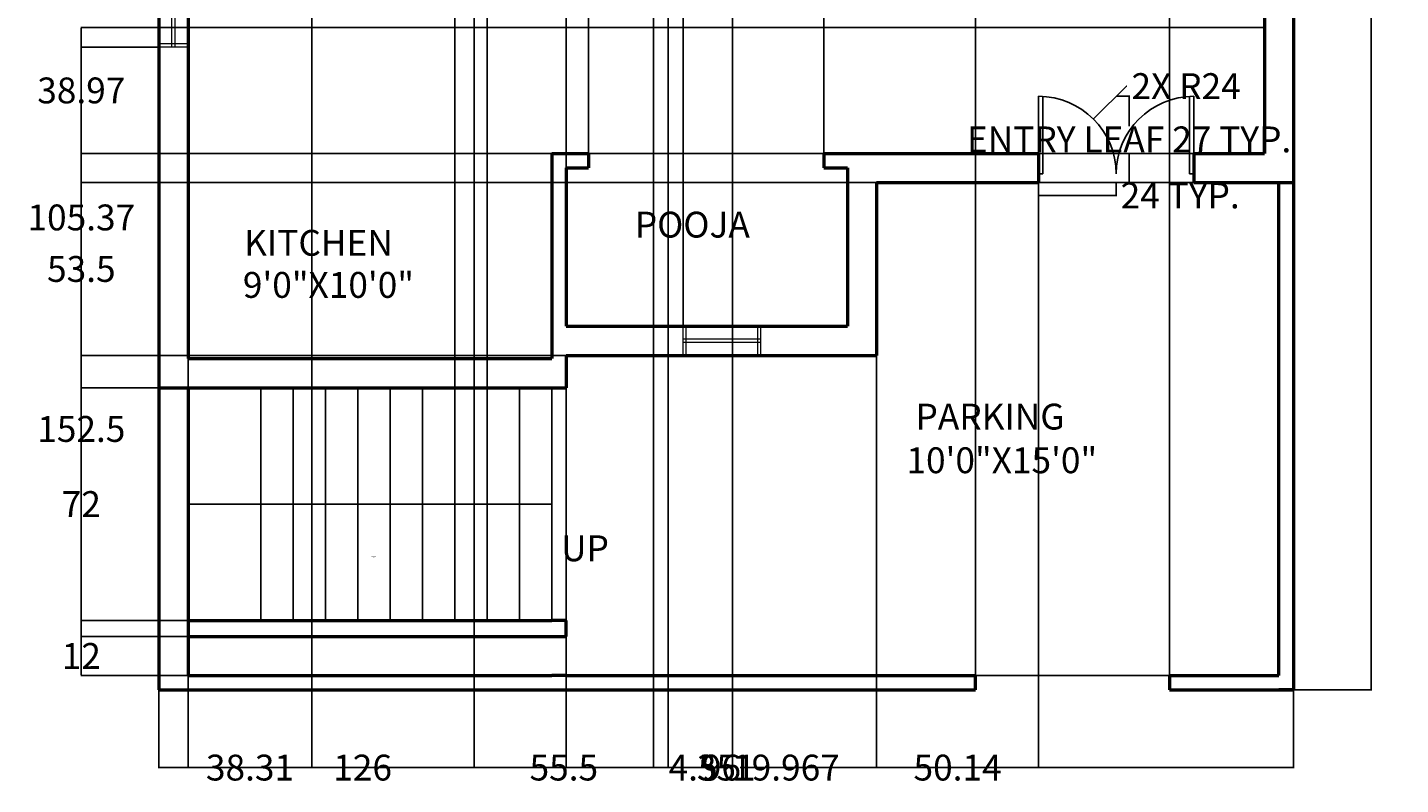
# Model space of a CAD drawing. Units: inches. Extents: x 16123781 to 16124206, y 158262361 to 158262900.
# Tile 1 of 2: x 16123781 to 16124206, y 158262361 to 158262596. Entities that reach past the tile are written whole.
import ezdxf

# ---------------------------------------------------------------- set-up
doc = ezdxf.new("R2010")
doc.units = ezdxf.units.IN
for name, color, linetype, lineweight in [('A-ANNO-DIMS', 2, 'Continuous', 18), ('A-ANNO-SYMB', 7, 'Continuous', 18), ('A-ANNO-TEXT', 7, 'Continuous', 25), ('A-AREA-IDEN', 7, 'Continuous', 25), ('A-Door', 150, 'Continuous', 25), ('stair', 10, 'Continuous', 25), ('wall', 130, 'Continuous', 50), ('window', 80, 'Continuous', 18)]:
    doc.layers.add(name, color=color, linetype=linetype, lineweight=lineweight)
doc.styles.get("Standard").update_dxf_attribs({"font": 'arial.ttf', "height": 8})
doc.dimstyles.get("Standard").update_dxf_attribs({"dimtxt": 0.18, "dimasz": 0.18, "dimexe": 0.18, "dimexo": 0.0625, "dimgap": 0.09, "dimtad": 0, "dimtih": 1, "dimtoh": 1, "dimdec": 4, "dimzin": 0, "dimdsep": 46, "dimtxsty": 'Standard', "dimcen": 0.09, "dimadec": 0, "dimazin": 0, "dimtfac": 1, "dimtdec": 4, "dimtofl": 0, "dimtmove": 0, "dimatfit": 3, "dimfxl": 1, "dimtolj": 1, "dimtzin": 0, "dimarcsym": 0})

# ---------------------------------------------------------------- blocks, each defined once
blk = doc.blocks.new('WIN-48IN')
for p, q in [((0, 0), (0, 48)), ((0, 48), (9, 48)), ((0, 47), (9, 47)), ((4, 0), (4, 48)), ((5, 0), (5, 48)), ((9, 48), (9, 0)), ((9, 1), (0, 1)), ((9, 0), (0, 0))]:
    blk.add_line(p, q)
blk = doc.blocks.new('WIN-24IN')
for p, q in [((0, 9), (24, 9)), ((0, 0), (0, 9)), ((1, 0), (1, 9)), ((23, 9), (23, 0)), ((24, 9), (24, 0)), ((24, 5), (0, 5)), ((24, 4), (0, 4)), ((24, 0), (0, 0))]:
    blk.add_line(p, q)
blk = doc.blocks.new('DOOR-LEAF-24IN')
for p, q in [((0, 0), (0, 26.67)), ((1.33, 2.67), (1.33, 26.63)), ((0, 2.67), (1.33, 2.67)), ((0, 0), (0, 1.6))]:
    blk.add_line(p, q)
blk.add_arc((0, 2.67), 24, 0, 90)
blk = doc.blocks.new('*D15')
at = {"layer": 'A-ANNO-DIMS', "color": 0, "lineweight": -2, "transparency": 16777216}
for p, q in [((16124117.96, 158262574.23), (16124122.08, 158262574.23)), ((16124121.9, 158262574.05), (16124121.9, 158262565.01)), ((16124121.9, 158262547.74), (16124121.9, 158262556.79)), ((16124117.96, 158262547.56), (16124122.08, 158262547.56))]:
    blk.add_line(p, q, dxfattribs=at)
at = {"layer": 'A-ANNO-DIMS', "color": 0, "transparency": 16777216}
for points in [[(16124121.87, 158262574.05), (16124121.93, 158262574.05), (16124121.9, 158262574.23)], [(16124121.87, 158262547.74), (16124121.93, 158262547.74), (16124121.9, 158262547.56)]]:
    blk.add_solid(points, dxfattribs=at)
at = {"layer": 'Defpoints', "color": 0, "transparency": 16777216}
for p in [(16124117.9, 158262574.23), (16124121.9, 158262574.23), (16124117.9, 158262547.56)]:
    blk.add_point(p, dxfattribs=at)
at = {"layer": 'A-ANNO-DIMS', "color": 0, "transparency": 16777216, "insert": (16124121.9, 158262560.9), "char_height": 8, "attachment_point": 5}
blk.add_mtext('\\A1;ENTRY LEAF 27 TYP.', dxfattribs=at)
blk = doc.blocks.new('*D16')
at = {"layer": 'A-ANNO-DIMS', "color": 0, "lineweight": -2, "transparency": 16777216}
for p, q in [((16124093.9, 158262547.5), (16124093.9, 158262543.38)), ((16124117.9, 158262547.5), (16124117.9, 158262543.38)), ((16124094.08, 158262543.56), (16124117.72, 158262543.56)), ((16124117.9, 158262543.56), (16124118.08, 158262543.56))]:
    blk.add_line(p, q, dxfattribs=at)
at = {"layer": 'A-ANNO-DIMS', "color": 0, "transparency": 16777216}
for points in [[(16124094.08, 158262543.59), (16124094.08, 158262543.53), (16124093.9, 158262543.56)], [(16124117.72, 158262543.59), (16124117.72, 158262543.53), (16124117.9, 158262543.56)]]:
    blk.add_solid(points, dxfattribs=at)
at = {"layer": 'Defpoints', "color": 0, "transparency": 16777216}
for p in [(16124093.9, 158262547.56), (16124117.9, 158262547.56), (16124117.9, 158262543.56)]:
    blk.add_point(p, dxfattribs=at)
at = {"layer": 'A-ANNO-DIMS', "color": 0, "transparency": 16777216, "insert": (16124137.71, 158262543.56), "char_height": 8, "attachment_point": 5}
blk.add_mtext('\\A1;24 TYP.', dxfattribs=at)
blk = doc.blocks.new('*D17')
at = {"layer": 'A-ANNO-DIMS', "color": 0, "lineweight": -2, "transparency": 16777216}
for p, q in [((16123821.76, 158262390.5), (16123821.76, 158262366.35)), ((16124172.76, 158262390.5), (16124172.76, 158262366.35)), ((16123821.94, 158262366.53), (16123989.11, 158262366.53)), ((16124172.58, 158262366.53), (16124005.41, 158262366.53))]:
    blk.add_line(p, q, dxfattribs=at)
at = {"layer": 'A-ANNO-DIMS', "color": 0, "transparency": 16777216}
for points in [[(16123821.94, 158262366.56), (16123821.94, 158262366.5), (16123821.76, 158262366.53)], [(16124172.58, 158262366.56), (16124172.58, 158262366.5), (16124172.76, 158262366.53)]]:
    blk.add_solid(points, dxfattribs=at)
at = {"layer": 'Defpoints', "color": 0, "transparency": 16777216}
for p in [(16123821.76, 158262390.56), (16124172.76, 158262390.56), (16124172.76, 158262366.53)]:
    blk.add_point(p, dxfattribs=at)
at = {"layer": 'A-ANNO-DIMS', "color": 0, "transparency": 16777216, "insert": (16123997.26, 158262366.53), "char_height": 8, "attachment_point": 5}
blk.add_mtext('\\A1;351', dxfattribs=at)
blk = doc.blocks.new('*D18')
at = {"layer": 'A-ANNO-DIMS', "color": 0, "lineweight": -2, "transparency": 16777216}
for p, q in [((16124172.82, 158262870.56), (16124196.97, 158262870.56)), ((16124196.79, 158262870.38), (16124196.79, 158262634.74)), ((16124196.79, 158262390.74), (16124196.79, 158262626.39)), ((16124172.82, 158262390.56), (16124196.97, 158262390.56))]:
    blk.add_line(p, q, dxfattribs=at)
at = {"layer": 'A-ANNO-DIMS', "color": 0, "transparency": 16777216}
for points in [[(16124196.76, 158262870.38), (16124196.82, 158262870.38), (16124196.79, 158262870.56)], [(16124196.76, 158262390.74), (16124196.82, 158262390.74), (16124196.79, 158262390.56)]]:
    blk.add_solid(points, dxfattribs=at)
at = {"layer": 'Defpoints', "color": 0, "transparency": 16777216}
for p in [(16124172.76, 158262870.56), (16124196.79, 158262870.56), (16124172.76, 158262390.56)]:
    blk.add_point(p, dxfattribs=at)
at = {"layer": 'A-ANNO-DIMS', "color": 0, "transparency": 16777216, "insert": (16124196.79, 158262630.56), "char_height": 8, "attachment_point": 5}
blk.add_mtext('\\A1;480', dxfattribs=at)
blk = doc.blocks.new('*D19')
at = {"layer": 'A-ANNO-DIMS', "color": 0, "lineweight": -2, "transparency": 16777216}
for p, q in [((16124074.35, 158262390.63), (16124074.35, 158262894.77)), ((16124074.53, 158262894.59), (16124098.52, 158262894.59)), ((16124134.17, 158262894.59), (16124110.18, 158262894.59)), ((16124134.35, 158262390.63), (16124134.35, 158262894.77))]:
    blk.add_line(p, q, dxfattribs=at)
at = {"layer": 'A-ANNO-DIMS', "color": 0, "transparency": 16777216}
for points in [[(16124074.53, 158262894.62), (16124074.53, 158262894.56), (16124074.35, 158262894.59)], [(16124134.17, 158262894.62), (16124134.17, 158262894.56), (16124134.35, 158262894.59)]]:
    blk.add_solid(points, dxfattribs=at)
at = {"layer": 'Defpoints', "color": 0, "transparency": 16777216}
for p in [(16124134.35, 158262894.59), (16124074.35, 158262390.56), (16124134.35, 158262390.56)]:
    blk.add_point(p, dxfattribs=at)
at = {"layer": 'A-ANNO-DIMS', "color": 0, "transparency": 16777216, "insert": (16124104.35, 158262894.59), "char_height": 8, "attachment_point": 5}
blk.add_mtext('\\A1;60', dxfattribs=at)
blk = doc.blocks.new('*D20')
at = {"layer": 'A-ANNO-DIMS', "color": 0, "lineweight": -2, "transparency": 16777216}
for p, q in [((16124134.35, 158262390.63), (16124134.35, 158262894.77)), ((16124134.53, 158262894.59), (16124140.74, 158262894.59)), ((16124172.58, 158262894.59), (16124166.37, 158262894.59)), ((16124172.76, 158262390.63), (16124172.76, 158262894.77))]:
    blk.add_line(p, q, dxfattribs=at)
at = {"layer": 'A-ANNO-DIMS', "color": 0, "transparency": 16777216}
for points in [[(16124134.53, 158262894.62), (16124134.53, 158262894.56), (16124134.35, 158262894.59)], [(16124172.58, 158262894.62), (16124172.58, 158262894.56), (16124172.76, 158262894.59)]]:
    blk.add_solid(points, dxfattribs=at)
at = {"layer": 'Defpoints', "color": 0, "transparency": 16777216}
for p in [(16124172.76, 158262894.59), (16124134.35, 158262390.56), (16124172.76, 158262390.56)]:
    blk.add_point(p, dxfattribs=at)
at = {"layer": 'A-ANNO-DIMS', "color": 0, "transparency": 16777216, "insert": (16124153.55, 158262894.59), "char_height": 8, "attachment_point": 5}
blk.add_mtext('\\A1;38.41', dxfattribs=at)
blk = doc.blocks.new('*D21')
at = {"layer": 'A-ANNO-DIMS', "color": 0, "lineweight": -2, "transparency": 16777216}
for p, q in [((16123821.76, 158262484), (16123821.76, 158262366.35)), ((16123947.76, 158262484), (16123947.76, 158262366.35)), ((16123821.94, 158262366.53), (16123876.21, 158262366.53)), ((16123947.58, 158262366.53), (16123893.31, 158262366.53))]:
    blk.add_line(p, q, dxfattribs=at)
at = {"layer": 'A-ANNO-DIMS', "color": 0, "transparency": 16777216}
for points in [[(16123821.94, 158262366.56), (16123821.94, 158262366.5), (16123821.76, 158262366.53)], [(16123947.58, 158262366.56), (16123947.58, 158262366.5), (16123947.76, 158262366.53)]]:
    blk.add_solid(points, dxfattribs=at)
at = {"layer": 'Defpoints', "color": 0, "transparency": 16777216}
for p in [(16123821.76, 158262484.06), (16123947.76, 158262484.06), (16123947.76, 158262366.53)]:
    blk.add_point(p, dxfattribs=at)
at = {"layer": 'A-ANNO-DIMS', "color": 0, "transparency": 16777216, "insert": (16123884.76, 158262366.53), "char_height": 8, "attachment_point": 5}
blk.add_mtext('\\A1;126', dxfattribs=at)
blk = doc.blocks.new('*D22')
at = {"layer": 'A-ANNO-DIMS', "color": 0, "lineweight": -2, "transparency": 16777216}
for p, q in [((16123947.76, 158262494), (16123947.76, 158262366.35)), ((16124043.76, 158262494), (16124043.76, 158262366.35)), ((16123947.94, 158262366.53), (16123989.94, 158262366.53)), ((16124043.58, 158262366.53), (16124001.58, 158262366.53))]:
    blk.add_line(p, q, dxfattribs=at)
at = {"layer": 'A-ANNO-DIMS', "color": 0, "transparency": 16777216}
for points in [[(16123947.94, 158262366.56), (16123947.94, 158262366.5), (16123947.76, 158262366.53)], [(16124043.58, 158262366.56), (16124043.58, 158262366.5), (16124043.76, 158262366.53)]]:
    blk.add_solid(points, dxfattribs=at)
at = {"layer": 'Defpoints', "color": 0, "transparency": 16777216}
for p in [(16123947.76, 158262494.06), (16124043.76, 158262494.06), (16124043.76, 158262366.53)]:
    blk.add_point(p, dxfattribs=at)
at = {"layer": 'A-ANNO-DIMS', "color": 0, "transparency": 16777216, "insert": (16123995.76, 158262366.53), "char_height": 8, "attachment_point": 5}
blk.add_mtext('\\A1;96', dxfattribs=at)
blk = doc.blocks.new('*D23')
at = {"layer": 'A-ANNO-DIMS', "color": 0, "lineweight": -2, "transparency": 16777216}
for p, q in [((16123947.76, 158262503.13), (16123947.76, 158262894.77)), ((16123947.94, 158262894.59), (16123952.22, 158262894.59)), ((16123983.73, 158262894.59), (16123979.45, 158262894.59)), ((16123983.91, 158262503.13), (16123983.91, 158262894.77))]:
    blk.add_line(p, q, dxfattribs=at)
at = {"layer": 'A-ANNO-DIMS', "color": 0, "transparency": 16777216}
for points in [[(16123947.94, 158262894.62), (16123947.94, 158262894.56), (16123947.76, 158262894.59)], [(16123983.73, 158262894.62), (16123983.73, 158262894.56), (16123983.91, 158262894.59)]]:
    blk.add_solid(points, dxfattribs=at)
at = {"layer": 'Defpoints', "color": 0, "transparency": 16777216}
for p in [(16123983.91, 158262894.59), (16123947.76, 158262503.06), (16123983.91, 158262503.06)]:
    blk.add_point(p, dxfattribs=at)
at = {"layer": 'A-ANNO-DIMS', "color": 0, "transparency": 16777216, "insert": (16123965.84, 158262894.59), "char_height": 8, "attachment_point": 5}
blk.add_mtext('\\A1;36.15', dxfattribs=at)
blk = doc.blocks.new('*D24')
at = {"layer": 'A-ANNO-DIMS', "color": 0, "lineweight": -2, "transparency": 16777216}
for p, q in [((16123830.7, 158262407.06), (16123797.55, 158262407.06)), ((16123797.73, 158262406.88), (16123797.73, 158262405.17)), ((16123797.73, 158262395.24), (16123797.73, 158262396.96)), ((16123830.7, 158262395.06), (16123797.55, 158262395.06))]:
    blk.add_line(p, q, dxfattribs=at)
at = {"layer": 'A-ANNO-DIMS', "color": 0, "transparency": 16777216}
for points in [[(16123797.7, 158262406.88), (16123797.76, 158262406.88), (16123797.73, 158262407.06)], [(16123797.7, 158262395.24), (16123797.76, 158262395.24), (16123797.73, 158262395.06)]]:
    blk.add_solid(points, dxfattribs=at)
at = {"layer": 'Defpoints', "color": 0, "transparency": 16777216}
for p in [(16123797.73, 158262407.06), (16123830.76, 158262407.06), (16123830.76, 158262395.06)]:
    blk.add_point(p, dxfattribs=at)
at = {"layer": 'A-ANNO-DIMS', "color": 0, "transparency": 16777216, "insert": (16123797.73, 158262401.06), "char_height": 8, "attachment_point": 5}
blk.add_mtext('\\A1;12', dxfattribs=at)
blk = doc.blocks.new('*D25')
at = {"layer": 'A-ANNO-DIMS', "color": 0, "lineweight": -2, "transparency": 16777216}
for p, q in [((16124043.7, 158262547.56), (16123797.55, 158262547.56)), ((16123797.73, 158262547.38), (16123797.73, 158262524.99)), ((16123797.73, 158262494.24), (16123797.73, 158262516.64)), ((16124043.7, 158262494.06), (16123797.55, 158262494.06))]:
    blk.add_line(p, q, dxfattribs=at)
at = {"layer": 'A-ANNO-DIMS', "color": 0, "transparency": 16777216}
for points in [[(16123797.7, 158262547.38), (16123797.76, 158262547.38), (16123797.73, 158262547.56)], [(16123797.7, 158262494.24), (16123797.76, 158262494.24), (16123797.73, 158262494.06)]]:
    blk.add_solid(points, dxfattribs=at)
at = {"layer": 'Defpoints', "color": 0, "transparency": 16777216}
for p in [(16123797.73, 158262547.56), (16124043.76, 158262547.56), (16124043.76, 158262494.06)]:
    blk.add_point(p, dxfattribs=at)
at = {"layer": 'A-ANNO-DIMS', "color": 0, "transparency": 16777216, "insert": (16123797.73, 158262520.81), "char_height": 8, "attachment_point": 5}
blk.add_mtext('\\A1;53.5', dxfattribs=at)
blk = doc.blocks.new('*D26')
at = {"layer": 'A-ANNO-DIMS', "color": 0, "lineweight": -2, "transparency": 16777216}
for p, q in [((16124168.2, 158262547.56), (16123797.55, 158262547.56)), ((16123797.73, 158262547.38), (16123797.73, 158262475.49)), ((16123797.73, 158262395.24), (16123797.73, 158262467.14)), ((16124168.2, 158262395.06), (16123797.55, 158262395.06))]:
    blk.add_line(p, q, dxfattribs=at)
at = {"layer": 'A-ANNO-DIMS', "color": 0, "transparency": 16777216}
for points in [[(16123797.7, 158262547.38), (16123797.76, 158262547.38), (16123797.73, 158262547.56)], [(16123797.7, 158262395.24), (16123797.76, 158262395.24), (16123797.73, 158262395.06)]]:
    blk.add_solid(points, dxfattribs=at)
at = {"layer": 'Defpoints', "color": 0, "transparency": 16777216}
for p in [(16123797.73, 158262547.56), (16124168.26, 158262547.56), (16124168.26, 158262395.06)]:
    blk.add_point(p, dxfattribs=at)
at = {"layer": 'A-ANNO-DIMS', "color": 0, "transparency": 16777216, "insert": (16123797.73, 158262471.31), "char_height": 8, "attachment_point": 5}
blk.add_mtext('\\A1;152.5', dxfattribs=at)
blk = doc.blocks.new('*D27')
at = {"layer": 'A-ANNO-DIMS', "color": 0, "lineweight": -2, "transparency": 16777216}
for p, q in [((16124043.76, 158262547.5), (16124043.76, 158262366.35)), ((16124093.9, 158262547.5), (16124093.9, 158262366.35)), ((16124043.94, 158262366.53), (16124055.26, 158262366.53)), ((16124093.72, 158262366.53), (16124082.4, 158262366.53))]:
    blk.add_line(p, q, dxfattribs=at)
at = {"layer": 'A-ANNO-DIMS', "color": 0, "transparency": 16777216}
for points in [[(16124043.94, 158262366.56), (16124043.94, 158262366.5), (16124043.76, 158262366.53)], [(16124093.72, 158262366.56), (16124093.72, 158262366.5), (16124093.9, 158262366.53)]]:
    blk.add_solid(points, dxfattribs=at)
at = {"layer": 'Defpoints', "color": 0, "transparency": 16777216}
for p in [(16124043.76, 158262547.56), (16124093.9, 158262547.56), (16124093.9, 158262366.53)]:
    blk.add_point(p, dxfattribs=at)
at = {"layer": 'A-ANNO-DIMS', "color": 0, "transparency": 16777216, "insert": (16124068.83, 158262366.53), "char_height": 8, "attachment_point": 5}
blk.add_mtext('\\A1;50.14', dxfattribs=at)
blk = doc.blocks.new('*D28')
at = {"layer": 'A-ANNO-DIMS', "color": 0, "lineweight": -2, "transparency": 16777216}
for p, q in [((16123821.7, 158262589.43), (16123797.55, 158262589.43)), ((16123797.73, 158262589.25), (16123797.73, 158262540.92)), ((16123797.73, 158262484.24), (16123797.73, 158262532.57)), ((16123821.7, 158262484.06), (16123797.55, 158262484.06))]:
    blk.add_line(p, q, dxfattribs=at)
at = {"layer": 'A-ANNO-DIMS', "color": 0, "transparency": 16777216}
for points in [[(16123797.7, 158262589.25), (16123797.76, 158262589.25), (16123797.73, 158262589.43)], [(16123797.7, 158262484.24), (16123797.76, 158262484.24), (16123797.73, 158262484.06)]]:
    blk.add_solid(points, dxfattribs=at)
at = {"layer": 'Defpoints', "color": 0, "transparency": 16777216}
for p in [(16123797.73, 158262589.43), (16123821.76, 158262589.43), (16123821.76, 158262484.06)]:
    blk.add_point(p, dxfattribs=at)
at = {"layer": 'A-ANNO-DIMS', "color": 0, "transparency": 16777216, "insert": (16123797.73, 158262536.75), "char_height": 8, "attachment_point": 5}
blk.add_mtext('\\A1;105.37', dxfattribs=at)
blk = doc.blocks.new('*D31')
at = {"layer": 'A-ANNO-DIMS', "color": 0, "lineweight": -2, "transparency": 16777216}
for p, q in [((16124163.7, 158262595.53), (16123797.55, 158262595.53)), ((16123797.73, 158262595.35), (16123797.73, 158262580.23)), ((16123797.73, 158262556.74), (16123797.73, 158262571.87)), ((16124163.7, 158262556.56), (16123797.55, 158262556.56))]:
    blk.add_line(p, q, dxfattribs=at)
at = {"layer": 'A-ANNO-DIMS', "color": 0, "transparency": 16777216}
for points in [[(16123797.7, 158262595.35), (16123797.76, 158262595.35), (16123797.73, 158262595.53)], [(16123797.7, 158262556.74), (16123797.76, 158262556.74), (16123797.73, 158262556.56)]]:
    blk.add_solid(points, dxfattribs=at)
at = {"layer": 'Defpoints', "color": 0, "transparency": 16777216}
for p in [(16123797.73, 158262595.53), (16124163.76, 158262595.53), (16124163.76, 158262556.56)]:
    blk.add_point(p, dxfattribs=at)
at = {"layer": 'A-ANNO-DIMS', "color": 0, "transparency": 16777216, "insert": (16123797.73, 158262576.05), "char_height": 8, "attachment_point": 5}
blk.add_mtext('\\A1;38.97', dxfattribs=at)
blk = doc.blocks.new('*D34')
at = {"layer": 'A-ANNO-DIMS', "color": 0, "lineweight": -2, "transparency": 16777216}
for p, q in [((16123830.7, 158262484.06), (16123797.55, 158262484.06)), ((16123797.73, 158262483.88), (16123797.73, 158262452.17)), ((16123797.73, 158262412.24), (16123797.73, 158262443.96)), ((16123830.7, 158262412.06), (16123797.55, 158262412.06))]:
    blk.add_line(p, q, dxfattribs=at)
at = {"layer": 'A-ANNO-DIMS', "color": 0, "transparency": 16777216}
for points in [[(16123797.7, 158262483.88), (16123797.76, 158262483.88), (16123797.73, 158262484.06)], [(16123797.7, 158262412.24), (16123797.76, 158262412.24), (16123797.73, 158262412.06)]]:
    blk.add_solid(points, dxfattribs=at)
at = {"layer": 'Defpoints', "color": 0, "transparency": 16777216}
for p in [(16123797.73, 158262484.06), (16123830.76, 158262484.06), (16123830.76, 158262412.06)]:
    blk.add_point(p, dxfattribs=at)
at = {"layer": 'A-ANNO-DIMS', "color": 0, "transparency": 16777216, "insert": (16123797.73, 158262448.06), "char_height": 8, "attachment_point": 5}
blk.add_mtext('\\A1;72', dxfattribs=at)
blk = doc.blocks.new('*D35')
at = {"layer": 'A-ANNO-DIMS', "color": 0, "lineweight": -2, "transparency": 16777216}
for p, q in [((16123913.26, 158262484.13), (16123913.26, 158262894.77)), ((16123913.44, 158262894.59), (16123923.08, 158262894.59)), ((16123923.26, 158262484.13), (16123923.26, 158262894.77)), ((16123923.26, 158262894.59), (16123923.44, 158262894.59))]:
    blk.add_line(p, q, dxfattribs=at)
at = {"layer": 'A-ANNO-DIMS', "color": 0, "transparency": 16777216}
for points in [[(16123913.44, 158262894.62), (16123913.44, 158262894.56), (16123913.26, 158262894.59)], [(16123923.08, 158262894.62), (16123923.08, 158262894.56), (16123923.26, 158262894.59)]]:
    blk.add_solid(points, dxfattribs=at)
at = {"layer": 'Defpoints', "color": 0, "transparency": 16777216}
for p in [(16123923.26, 158262894.59), (16123913.26, 158262484.06), (16123923.26, 158262484.06)]:
    blk.add_point(p, dxfattribs=at)
at = {"layer": 'A-ANNO-DIMS', "color": 0, "transparency": 16777216, "insert": (16123928.87, 158262894.59), "char_height": 8, "attachment_point": 5}
blk.add_mtext('\\A1;10', dxfattribs=at)
blk = doc.blocks.new('*D36')
at = {"layer": 'A-ANNO-DIMS', "color": 0, "lineweight": -2, "transparency": 16777216}
for p, q in [((16123954.69, 158262552.13), (16123954.69, 158262894.77)), ((16123954.87, 158262894.59), (16123978.31, 158262894.59)), ((16124027.32, 158262894.59), (16124003.88, 158262894.59)), ((16124027.5, 158262552.13), (16124027.5, 158262894.77))]:
    blk.add_line(p, q, dxfattribs=at)
at = {"layer": 'A-ANNO-DIMS', "color": 0, "transparency": 16777216}
for points in [[(16123954.87, 158262894.62), (16123954.87, 158262894.56), (16123954.69, 158262894.59)], [(16124027.32, 158262894.62), (16124027.32, 158262894.56), (16124027.5, 158262894.59)]]:
    blk.add_solid(points, dxfattribs=at)
at = {"layer": 'Defpoints', "color": 0, "transparency": 16777216}
for p in [(16124027.5, 158262894.59), (16123954.69, 158262552.06), (16124027.5, 158262552.06)]:
    blk.add_point(p, dxfattribs=at)
at = {"layer": 'A-ANNO-DIMS', "color": 0, "transparency": 16777216, "insert": (16123991.1, 158262894.59), "char_height": 8, "attachment_point": 5}
blk.add_mtext('\\A1;72.81', dxfattribs=at)
blk = doc.blocks.new('*D37')
at = {"layer": 'A-ANNO-DIMS', "color": 0, "lineweight": -2, "transparency": 16777216}
for p, q in [((16123919.260748, 158262688.500323), (16123919.260748, 158262366.352823)), ((16123974.760748, 158262688.500323), (16123974.760748, 158262366.352823)), ((16123919.440748, 158262366.532823), (16123936.500557, 158262366.532823)), ((16123974.580748, 158262366.532823), (16123957.520939, 158262366.532823))]:
    blk.add_line(p, q, dxfattribs=at)
at = {"layer": 'A-ANNO-DIMS', "color": 0, "transparency": 16777216}
for points in [[(16123919.440748, 158262366.562823), (16123919.440748, 158262366.502823), (16123919.260748, 158262366.532823)], [(16123974.580748, 158262366.562823), (16123974.580748, 158262366.502823), (16123974.760748, 158262366.532823)]]:
    blk.add_solid(points, dxfattribs=at)
at = {"layer": 'Defpoints', "color": 0, "transparency": 16777216}
for p in [(16123919.260748, 158262688.562823), (16123974.760748, 158262688.562823), (16123974.760748, 158262366.532823)]:
    blk.add_point(p, dxfattribs=at)
at = {"layer": 'A-ANNO-DIMS', "color": 0, "transparency": 16777216, "insert": (16123947.010748, 158262366.532823), "char_height": 8, "attachment_point": 5}
blk.add_mtext('\\A1;55.5', dxfattribs=at)
blk = doc.blocks.new('*D39')
at = {"layer": 'A-ANNO-DIMS', "color": 0, "lineweight": -2, "transparency": 16777216}
for p, q in [((16123974.760748, 158262660.000323), (16123974.760748, 158262366.352823)), ((16123979.260748, 158262660.000323), (16123979.260748, 158262366.352823)), ((16123974.940748, 158262366.532823), (16123979.080748, 158262366.532823)), ((16123979.260748, 158262366.532823), (16123979.440748, 158262366.532823))]:
    blk.add_line(p, q, dxfattribs=at)
at = {"layer": 'A-ANNO-DIMS', "color": 0, "transparency": 16777216}
for points in [[(16123974.940748, 158262366.562823), (16123974.940748, 158262366.502823), (16123974.760748, 158262366.532823)], [(16123979.080748, 158262366.562823), (16123979.080748, 158262366.502823), (16123979.260748, 158262366.532823)]]:
    blk.add_solid(points, dxfattribs=at)
at = {"layer": 'Defpoints', "color": 0, "transparency": 16777216}
for p in [(16123974.760748, 158262660.062823), (16123979.260748, 158262660.062823), (16123979.260748, 158262366.532823)]:
    blk.add_point(p, dxfattribs=at)
at = {"layer": 'A-ANNO-DIMS', "color": 0, "transparency": 16777216, "insert": (16123987.004145, 158262366.532823), "char_height": 8, "attachment_point": 5}
blk.add_mtext('\\A1;4.5', dxfattribs=at)
blk = doc.blocks.new('*D40')
at = {"layer": 'A-ANNO-DIMS', "color": 0, "lineweight": -2, "transparency": 16777216}
for p, q in [((16123830.76, 158262724.5), (16123830.76, 158262366.35)), ((16123869.07, 158262724.5), (16123869.07, 158262366.35)), ((16123830.94, 158262366.53), (16123837.1, 158262366.53)), ((16123868.89, 158262366.53), (16123862.73, 158262366.53))]:
    blk.add_line(p, q, dxfattribs=at)
at = {"layer": 'A-ANNO-DIMS', "color": 0, "transparency": 16777216}
for points in [[(16123830.94, 158262366.56), (16123830.94, 158262366.5), (16123830.76, 158262366.53)], [(16123868.89, 158262366.56), (16123868.89, 158262366.5), (16123869.07, 158262366.53)]]:
    blk.add_solid(points, dxfattribs=at)
at = {"layer": 'Defpoints', "color": 0, "transparency": 16777216}
for p in [(16123830.76, 158262724.56), (16123869.07, 158262724.56), (16123869.07, 158262366.53)]:
    blk.add_point(p, dxfattribs=at)
at = {"layer": 'A-ANNO-DIMS', "color": 0, "transparency": 16777216, "insert": (16123849.92, 158262366.53), "char_height": 8, "attachment_point": 5}
blk.add_mtext('\\A1;38.31', dxfattribs=at)
blk = doc.blocks.new('*D41')
at = {"layer": 'A-ANNO-DIMS', "color": 0, "lineweight": -2, "transparency": 16777216}
for p, q in [((16123979.26, 158262777.5), (16123979.26, 158262366.35)), ((16123999.23, 158262777.5), (16123999.23, 158262366.35)), ((16123979.44, 158262366.53), (16123999.05, 158262366.53)), ((16123999.23, 158262366.53), (16123999.41, 158262366.53))]:
    blk.add_line(p, q, dxfattribs=at)
at = {"layer": 'A-ANNO-DIMS', "color": 0, "transparency": 16777216}
for points in [[(16123979.44, 158262366.56), (16123979.44, 158262366.5), (16123979.26, 158262366.53)], [(16123999.05, 158262366.56), (16123999.05, 158262366.5), (16123999.23, 158262366.53)]]:
    blk.add_solid(points, dxfattribs=at)
at = {"layer": 'Defpoints', "color": 0, "transparency": 16777216}
for p in [(16123979.26, 158262777.56), (16123999.23, 158262777.56), (16123999.23, 158262366.53)]:
    blk.add_point(p, dxfattribs=at)
at = {"layer": 'A-ANNO-DIMS', "color": 0, "transparency": 16777216, "insert": (16124015.73, 158262366.53), "char_height": 8, "attachment_point": 5}
blk.add_mtext('\\A1;19.967', dxfattribs=at)
blk = doc.blocks.new('*D46')
at = {"layer": 'A-ANNO-DIMS', "color": 0, "lineweight": -2, "transparency": 16777216}
for p, q in [((16124121.05, 158262577.38), (16124111, 158262567.33)), ((16124121.23, 158262577.38), (16124121.05, 158262577.38)), ((16124093.81, 158262550.23), (16124093.99, 158262550.23)), ((16124093.9, 158262550.14), (16124093.9, 158262550.32))]:
    blk.add_line(p, q, dxfattribs=at)
at = {"layer": 'A-ANNO-DIMS', "color": 0, "transparency": 16777216}
blk.add_solid([(16124110.98, 158262567.35), (16124111.02, 158262567.31), (16124110.87, 158262567.2)], dxfattribs=at)
at = {"layer": 'Defpoints', "color": 0, "transparency": 16777216}
for p in [(16124110.87, 158262567.2), (16124093.9, 158262550.23)]:
    blk.add_point(p, dxfattribs=at)
at = {"layer": 'A-ANNO-DIMS', "color": 0, "transparency": 16777216, "insert": (16124139.53, 158262577.38), "char_height": 8, "attachment_point": 5}
blk.add_mtext('\\A1;2X R24', dxfattribs=at)

msp = doc.modelspace()

# ---------------------------------------------------------------- linework, layer by layer
at = {"layer": 'A-ANNO-SYMB'}
msp.add_lwpolyline([(16123888.2553, 158262431.5958, 0, 5, 0), (16123900.5329, 158262431.831, 0, 0, 0), (16123943.2607, 158262431.831, 0, 0, 0)], format="xyseb", dxfattribs=at)
at = {"layer": 'stair'}
for p, q in [((16123853.2607, 158262484.0628), (16123853.2607, 158262412.0628)), ((16123863.2607, 158262484.0628), (16123863.2607, 158262412.0628)), ((16123873.2607, 158262484.0628), (16123873.2607, 158262412.0628)), ((16123883.2607, 158262484.0628), (16123883.2607, 158262412.0628)), ((16123893.2607, 158262484.0628), (16123893.2607, 158262412.0628)), ((16123903.2607, 158262484.0628), (16123903.2607, 158262412.0628)), ((16123913.2607, 158262484.0628), (16123913.2607, 158262412.0628)), ((16123923.2607, 158262484.0628), (16123923.2607, 158262412.0628)), ((16123933.2607, 158262484.0628), (16123933.2607, 158262412.0628)), ((16123943.2607, 158262484.0628), (16123943.2607, 158262412.0628)), ((16123943.2607, 158262448.0628), (16123830.7607, 158262448.0628))]:
    msp.add_line(p, q, dxfattribs=at)
at = {"layer": 'wall'}
for p, q in [((16123821.7607, 158262870.5628), (16123821.7607, 158262390.5628)), ((16124172.7607, 158262870.5628), (16124172.7607, 158262390.5628)), ((16124163.7607, 158262861.5628), (16124163.7607, 158262556.5628)), ((16123830.7607, 158262660.0628), (16123830.7607, 158262493.0628)), ((16123943.2607, 158262556.5628), (16123954.6914, 158262556.5628)), ((16123943.2607, 158262556.5628), (16123943.2607, 158262493.0628)), ((16123954.6914, 158262556.5628), (16123954.6914, 158262552.0628)), ((16124027.5035, 158262556.5628), (16124027.5035, 158262552.0628)), ((16124027.5035, 158262556.5628), (16124093.9003, 158262556.5628)), ((16124093.9003, 158262556.5628), (16124093.9003, 158262547.5628)), ((16124141.9003, 158262556.5628), (16124141.9003, 158262547.5628)), ((16124141.9003, 158262556.5628), (16124163.7607, 158262556.5628)), ((16123947.7607, 158262552.0628), (16123954.6914, 158262552.0628)), ((16123947.7607, 158262552.0628), (16123947.7607, 158262503.0628)), ((16124027.5035, 158262552.0628), (16124034.7607, 158262552.0628)), ((16124034.7607, 158262552.0628), (16124034.7607, 158262503.0628)), ((16124043.7607, 158262547.5628), (16124043.7607, 158262494.0628)), ((16124043.7607, 158262547.5628), (16124093.9003, 158262547.5628)), ((16124141.9003, 158262547.5628), (16124172.7607, 158262547.5628)), ((16124168.2607, 158262395.0628), (16124168.2607, 158262547.5628)), ((16123947.7607, 158262503.0628), (16124034.7607, 158262503.0628)), ((16123947.7607, 158262494.0628), (16124043.7607, 158262494.0628)), ((16123947.7607, 158262494.0628), (16123947.7607, 158262484.0628)), ((16123830.7607, 158262493.0628), (16123943.2607, 158262493.0628)), ((16123821.7607, 158262484.0628), (16123947.7607, 158262484.0628)), ((16123830.7607, 158262484.0628), (16123830.7607, 158262395.0628)), ((16123830.7607, 158262412.0628), (16123943.2607, 158262412.0628)), ((16123947.7607, 158262412.0628), (16123943.2607, 158262412.0628)), ((16123947.7607, 158262407.0628), (16123947.7607, 158262412.0628)), ((16123830.7607, 158262407.0628), (16123947.7607, 158262407.0628)), ((16123830.7607, 158262395.0628), (16123943.2607, 158262395.0628)), ((16123947.7607, 158262395.0628), (16123943.2607, 158262395.0628)), ((16123947.7607, 158262395.0628), (16124074.3474, 158262395.0628)), ((16124134.3474, 158262395.0628), (16124168.2607, 158262395.0628)), ((16123821.7607, 158262390.5628), (16124074.3474, 158262390.5628)), ((16124134.3474, 158262390.5628), (16124172.7607, 158262390.5628)), ((16124172.7607, 158262390.5628), (16124168.2607, 158262390.5628))]:
    msp.add_line(p, q, dxfattribs=at)
for points in [[(16124074.3474, 158262390.5628), (16124074.3474, 158262395.0628)], [(16124134.3474, 158262395.0628), (16124134.3474, 158262390.5628)]]:
    msp.add_lwpolyline(points, dxfattribs=at)

# ---------------------------------------------------------------- block references
at = {"layer": 'A-Door'}
msp.add_blockref('DOOR-LEAF-24IN', (16124093.9, 158262547.563), dxfattribs=at)
at = {"layer": 'A-Door', "extrusion": (0, 0, -1), "zscale": -1}
msp.add_blockref('DOOR-LEAF-24IN', (-16124141.9006, 158262547.563), dxfattribs=at)
at = {"layer": 'window'}
for name, p in [('WIN-48IN', (16123821.761, 158262589.4304)), ('WIN-24IN', (16123983.9096, 158262494.063))]:
    msp.add_blockref(name, p, dxfattribs=at)

# ---------------------------------------------------------------- texts
at = {"layer": 'A-ANNO-TEXT'}
msp.add_text('UP', height=8, dxfattribs=at).set_placement((16123946.1837, 158262430.382))
at = {"layer": 'A-AREA-IDEN'}
for s, p in [('POOJA', (16123968.974, 158262530.5227)), ('KITCHEN', (16123848.1057, 158262524.8895)), (' 9\'0"X10\'0"', (16123845.2684, 158262511.8763)), ('PARKING ', (16124055.8144, 158262471.1223)), ('10\'0"X15\'0"', (16124053.011, 158262457.6206))]:
    msp.add_text(s, height=8, dxfattribs=at).set_placement(p)

# ---------------------------------------------------------------- dimensions: what is measured, and where the dimension line sits
at = {"layer": 'A-ANNO-DIMS'}
for base, p1, p2, override, picture, middle in [((16123923.2607, 158262894.5928), (16123913.2607, 158262484.0628), (16123923.2607, 158262484.0628), {"dimdec": 0, "dimlfac": 1, "dimrnd": 0, "dimzin": 0, "dimdsep": 46, "dimlunit": 2}, '*D35', (16123928.8704, 158262894.5928)), ((16123983.9094, 158262894.5928), (16123947.7607, 158262503.0628), (16123983.9094, 158262503.0628), {"dimdec": 2, "dimlfac": 1, "dimrnd": 0, "dimzin": 0, "dimdsep": 46, "dimlunit": 2}, '*D23', (16123965.8351, 158262894.5928)), ((16124027.5035, 158262894.5928), (16123954.6914, 158262552.0628), (16124027.5035, 158262552.0628), {"dimdec": 2, "dimlfac": 1, "dimrnd": 0, "dimzin": 0, "dimdsep": 46, "dimlunit": 2}, '*D36', (16123991.0974, 158262894.5928)), ((16124134.3474, 158262894.5928), (16124074.3474, 158262390.5628), (16124134.3474, 158262390.5628), {"dimdec": 0, "dimlfac": 1, "dimrnd": 0, "dimzin": 0, "dimdsep": 46, "dimlunit": 2}, '*D19', (16124104.3474, 158262894.5928)), ((16124172.7607, 158262894.5928), (16124134.3474, 158262390.5628), (16124172.7607, 158262390.5628), {"dimdec": 2, "dimlfac": 1, "dimrnd": 0, "dimzin": 0, "dimdsep": 46, "dimlunit": 2}, '*D20', (16124153.5541, 158262894.5928)), ((16123999.2274, 158262366.5328), (16123979.2607, 158262777.5628), (16123999.2274, 158262777.5628), {"dimdec": 3, "dimlfac": 1, "dimrnd": 0, "dimzin": 0, "dimdsep": 46, "dimlunit": 2}, '*D41', (16124015.7265, 158262366.5328)), ((16123869.0741, 158262366.5328), (16123830.7607, 158262724.5628), (16123869.0741, 158262724.5628), {"dimdec": 2, "dimlfac": 1, "dimrnd": 0, "dimzin": 0, "dimdsep": 46, "dimlunit": 2}, '*D40', (16123849.9174, 158262366.5328)), ((16123974.7607, 158262366.5328), (16123919.2607, 158262688.5628), (16123974.7607, 158262688.5628), {"dimdec": 1, "dimlfac": 1, "dimrnd": 0, "dimzin": 0, "dimdsep": 46, "dimlunit": 2}, '*D37', (16123947.0107, 158262366.5328)), ((16123979.2607, 158262366.5328), (16123974.7607, 158262660.0628), (16123979.2607, 158262660.0628), {"dimdec": 1, "dimlfac": 1, "dimrnd": 0, "dimzin": 0, "dimdsep": 46, "dimlunit": 2}, '*D39', (16123987.0041, 158262366.5328)), ((16124093.9003, 158262366.5328), (16124043.7607, 158262547.5628), (16124093.9003, 158262547.5628), {"dimdec": 2, "dimlfac": 1, "dimrnd": 0, "dimzin": 0, "dimdsep": 46, "dimlunit": 2}, '*D27', (16124068.8305, 158262366.5328)), ((16124043.7607, 158262366.5328), (16123947.7607, 158262494.0628), (16124043.7607, 158262494.0628), {"dimdec": 0, "dimlfac": 1, "dimrnd": 0, "dimzin": 0, "dimdsep": 46, "dimlunit": 2}, '*D22', (16123995.7607, 158262366.5328)), ((16123947.7607, 158262366.5328), (16123821.7607, 158262484.0628), (16123947.7607, 158262484.0628), {"dimdec": 0, "dimlfac": 1, "dimrnd": 0, "dimzin": 0, "dimdsep": 46, "dimlunit": 2}, '*D21', (16123884.7607, 158262366.5328)), ((16124172.7607, 158262366.5328), (16123821.7607, 158262390.5628), (16124172.7607, 158262390.5628), {"dimdec": 0, "dimlfac": 1, "dimrnd": 0, "dimzin": 0, "dimdsep": 46, "dimlunit": 2}, '*D17', (16123997.2607, 158262366.5328))]:
    dim = msp.add_linear_dim(base=base, p1=p1, p2=p2, dimstyle='Standard', override=override, dxfattribs=at)
    dim.commit()
    dim.dimension.update_dxf_attribs({"geometry": picture, "text_midpoint": middle})
for base, p1, p2, override, picture, middle in [((16124196.7907, 158262870.5628), (16124172.7607, 158262390.5628), (16124172.7607, 158262870.5628), {"dimdec": 0, "dimlfac": 1, "dimrnd": 0, "dimzin": 0, "dimdsep": 46, "dimlunit": 2}, '*D18', (16124196.7907, 158262630.5628)), ((16123797.7307, 158262595.5349), (16124163.7607, 158262556.5628), (16124163.7607, 158262595.5349), {"dimdec": 2, "dimlfac": 1, "dimrnd": 0, "dimzin": 0, "dimdsep": 46, "dimlunit": 2}, '*D31', (16123797.7307, 158262576.0489)), ((16123797.7307, 158262589.4303), (16123821.7607, 158262484.0628), (16123821.7607, 158262589.4303), {"dimdec": 2, "dimlfac": 1, "dimrnd": 0, "dimzin": 0, "dimdsep": 46, "dimlunit": 2}, '*D28', (16123797.7307, 158262536.7465)), ((16123797.7307, 158262547.5628), (16124168.2607, 158262395.0628), (16124168.2607, 158262547.5628), {"dimdec": 1, "dimlfac": 1, "dimrnd": 0, "dimzin": 0, "dimdsep": 46, "dimlunit": 2}, '*D26', (16123797.7307, 158262471.3128)), ((16123797.7307, 158262547.5628), (16124043.7607, 158262494.0628), (16124043.7607, 158262547.5628), {"dimdec": 1, "dimlfac": 1, "dimrnd": 0, "dimzin": 0, "dimdsep": 46, "dimlunit": 2}, '*D25', (16123797.7307, 158262520.8128)), ((16123797.7307, 158262484.0628), (16123830.7607, 158262412.0628), (16123830.7607, 158262484.0628), {"dimdec": 0, "dimlfac": 1, "dimrnd": 0, "dimzin": 0, "dimdsep": 46, "dimlunit": 2}, '*D34', (16123797.7307, 158262448.0628)), ((16123797.7307, 158262407.0628), (16123830.7607, 158262395.0628), (16123830.7607, 158262407.0628), {"dimdec": 0, "dimlfac": 1, "dimrnd": 0, "dimzin": 0, "dimdsep": 46, "dimlunit": 2}, '*D24', (16123797.7307, 158262401.0628))]:
    dim = msp.add_linear_dim(base=base, p1=p1, p2=p2, angle=90, dimstyle='Standard', override=override, dxfattribs=at)
    dim.commit()
    dim.dimension.update_dxf_attribs({"geometry": picture, "text_midpoint": middle})
dim = msp.add_radius_dim(center=(16124093.9003, 158262550.2295), mpoint=(16124110.871, 158262567.2), text='2X <>', dimstyle='Standard', override={"dimdec": 0, "dimlfac": 1, "dimrnd": 0, "dimzin": 0, "dimdsep": 46, "dimlunit": 2}, dxfattribs=at)
dim.commit()
dim.dimension.update_dxf_attribs({"geometry": '*D46', "text_midpoint": (16124139.528, 158262577.3822), "dimtype": 164})
dim = msp.add_linear_dim(base=(16124121.9003, 158262574.2295), p1=(16124117.9003, 158262547.5628), p2=(16124117.9003, 158262574.2295), angle=90, text='ENTRY LEAF <> TYP.', dimstyle='Standard', override={"dimdec": 0, "dimlfac": 1, "dimrnd": 0, "dimzin": 0, "dimdsep": 46, "dimlunit": 2}, dxfattribs=at)
dim.commit()
dim.dimension.update_dxf_attribs({"geometry": '*D15', "text_midpoint": (16124121.9003, 158262560.8962)})
dim = msp.add_linear_dim(base=(16124117.9003, 158262543.5628), p1=(16124093.9003, 158262547.5628), p2=(16124117.9003, 158262547.5628), text='<> TYP.', dimstyle='Standard', override={"dimdec": 0, "dimlfac": 1, "dimrnd": 0, "dimzin": 0, "dimdsep": 46, "dimlunit": 2}, dxfattribs=at)
dim.commit()
dim.dimension.update_dxf_attribs({"geometry": '*D16', "text_midpoint": (16124137.7092, 158262543.5628)})

doc.saveas('drawing.dxf')
